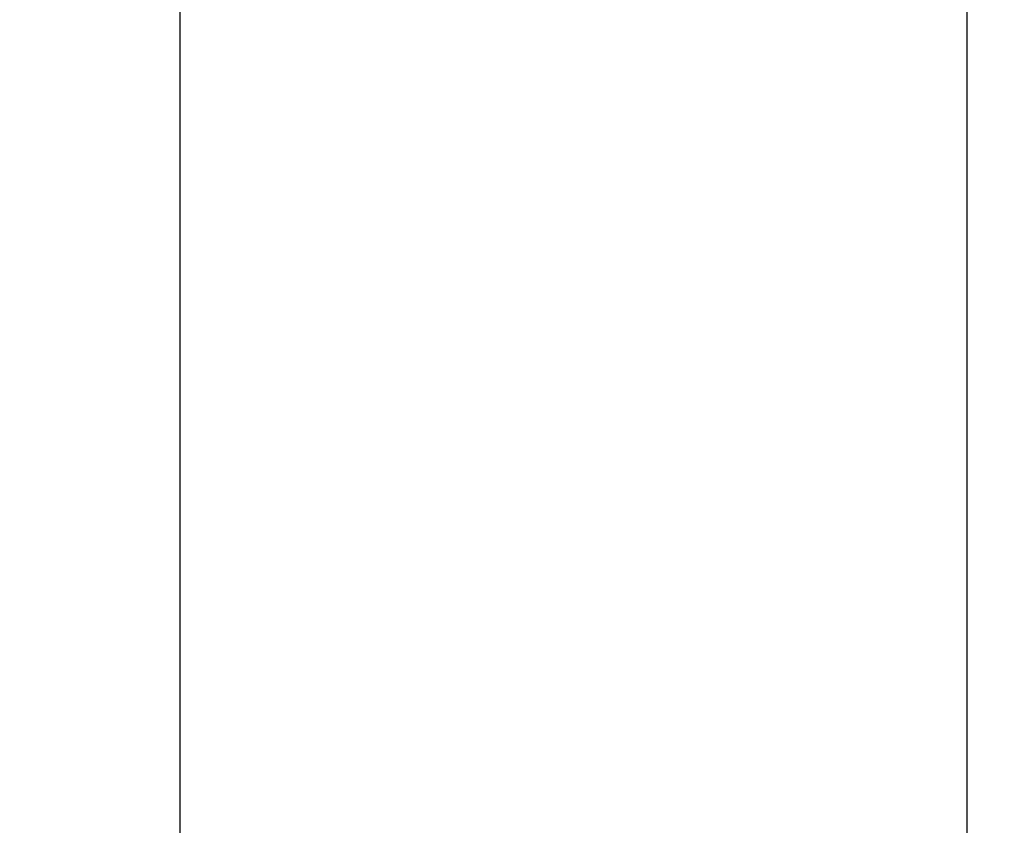
# Model space of a CAD drawing. Units: inches. Extents: x 2091 to 2899, y 967 to 2217.
# Tile 19 of 256: x 2351 to 2390, y 1032 to 1064. Entities that reach past the tile are written whole.
import ezdxf

# ---------------------------------------------------------------- set-up
doc = ezdxf.new("R2010")
doc.units = ezdxf.units.IN
doc.layers.add('A-ANNO-DIMS', color=2, linetype='Continuous', lineweight=18)
doc.styles.get("Standard").update_dxf_attribs({"font": 'arial.ttf'})
doc.dimstyles.new('ISO-25', dxfattribs={"dimtxt": 4, "dimasz": 4, "dimexe": 1.25, "dimexo": 0.625, "dimtad": 1, "dimdec": 0, "dimlunit": 3, "dimtxsty": 'Standard', "dimcen": 2.5, "dimadec": 0, "dimazin": 0, "dimtfac": 1, "dimtdec": 0, "dimtmove": 0, "dimatfit": 3, "dimfxl": 1, "dimarcsym": 0})

# ---------------------------------------------------------------- blocks, each defined once
blk = doc.blocks.new('*D68')
at = {"layer": 'A-ANNO-DIMS', "color": 0, "lineweight": -2, "transparency": 16777216}
for p, q in [((2317.144, 1535.794), (2317.144, 969.464)), ((2459.384, 1535.794), (2459.384, 969.464)), ((2321.144, 970.714), (2455.384, 970.714))]:
    blk.add_line(p, q, dxfattribs=at)
at = {"layer": 'A-ANNO-DIMS', "color": 0, "transparency": 16777216}
for points in [[(2321.144, 971.381), (2321.144, 970.048), (2317.144, 970.714)], [(2455.384, 971.381), (2455.384, 970.048), (2459.384, 970.714)]]:
    blk.add_solid(points, dxfattribs=at)
at = {"layer": 'Defpoints', "color": 0, "transparency": 16777216}
for p in [(2317.144, 1536.419), (2459.384, 1536.419), (2459.384, 970.714)]:
    blk.add_point(p, dxfattribs=at)
at = {"layer": 'A-ANNO-DIMS', "color": 0, "transparency": 16777216, "insert": (2388.264, 973.382), "char_height": 4, "attachment_point": 5}
blk.add_mtext('11\'-10"', dxfattribs=at)
blk = doc.blocks.new('*D71')
at = {"layer": 'A-ANNO-DIMS', "color": 0, "lineweight": -2, "transparency": 16777216}
for p, q in [((2212.144, 1351.294), (2212.144, 969.464)), ((2452.144, 1351.294), (2452.144, 969.464)), ((2216.144, 970.714), (2448.144, 970.714))]:
    blk.add_line(p, q, dxfattribs=at)
at = {"layer": 'A-ANNO-DIMS', "color": 0, "transparency": 16777216}
for points in [[(2216.144, 971.381), (2216.144, 970.048), (2212.144, 970.714)], [(2448.144, 971.381), (2448.144, 970.048), (2452.144, 970.714)]]:
    blk.add_solid(points, dxfattribs=at)
at = {"layer": 'Defpoints', "color": 0, "transparency": 16777216}
for p in [(2212.144, 1351.919), (2452.144, 1351.919), (2452.144, 970.714)]:
    blk.add_point(p, dxfattribs=at)
at = {"layer": 'A-ANNO-DIMS', "color": 0, "transparency": 16777216, "insert": (2332.144, 973.382), "char_height": 4, "attachment_point": 5}
blk.add_mtext('20\'-0"', dxfattribs=at)
blk = doc.blocks.new('*D82')
at = {"layer": 'A-ANNO-DIMS', "color": 0, "lineweight": -2, "transparency": 16777216}
for p, q in [((2357.434, 1549.361), (2357.434, 969.464)), ((2388.969, 1549.361), (2388.969, 969.464)), ((2361.434, 970.714), (2384.969, 970.714))]:
    blk.add_line(p, q, dxfattribs=at)
at = {"layer": 'A-ANNO-DIMS', "color": 0, "transparency": 16777216}
for points in [[(2361.434, 971.381), (2361.434, 970.048), (2357.434, 970.714)], [(2384.969, 971.381), (2384.969, 970.048), (2388.969, 970.714)]]:
    blk.add_solid(points, dxfattribs=at)
at = {"layer": 'Defpoints', "color": 0, "transparency": 16777216}
for p in [(2357.434, 1549.986), (2388.969, 1549.986), (2388.969, 970.714)]:
    blk.add_point(p, dxfattribs=at)
at = {"layer": 'A-ANNO-DIMS', "color": 0, "transparency": 16777216, "insert": (2373.202, 973.408), "char_height": 4, "attachment_point": 5}
blk.add_mtext('2\'-7 1/2"', dxfattribs=at)

msp = doc.modelspace()

# ---------------------------------------------------------------- dimensions: what is measured, and where the dimension line sits
at = {"layer": 'A-ANNO-DIMS'}
for base, p1, p2, picture, middle in [((2388.969, 970.714), (2357.434, 1549.986), (2388.969, 1549.986), '*D82', (2373.202, 973.408)), ((2459.384, 970.714), (2317.144, 1536.419), (2459.384, 1536.419), '*D68', (2388.264, 973.382)), ((2452.144, 970.714), (2212.144, 1351.919), (2452.144, 1351.919), '*D71', (2332.144, 973.382))]:
    dim = msp.add_linear_dim(base=base, p1=p1, p2=p2, dimstyle='ISO-25', override={"dimdec": 1, "dimlfac": 1, "dimrnd": 0, "dimzin": 1, "dimdsep": 46, "dimlunit": 4, "dimfrac": 2}, dxfattribs=at)
    dim.commit()
    dim.dimension.update_dxf_attribs({"geometry": picture, "text_midpoint": middle})

doc.saveas('drawing.dxf')
